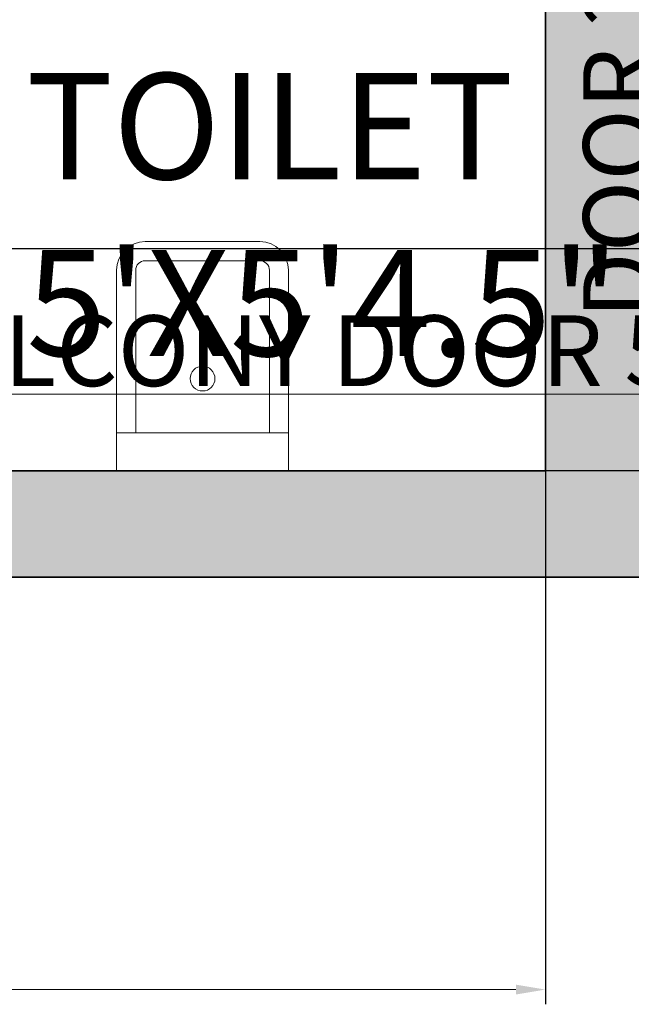
# Model space of a CAD drawing. Units: inches. Extents: x 2696 to 3240, y 1564 to 2310.
# Tile 11 of 76: x 2912 to 2964, y 1569 to 1652. Entities that reach past the tile are written whole.
import ezdxf

# ---------------------------------------------------------------- set-up
doc = ezdxf.new("R2010")
doc.units = ezdxf.units.IN
for name, color, linetype, lineweight in [('A-ANNO-DIMS', 3, 'Continuous', 18), ('A-AREA-IDEN', 7, 'Continuous', 18), ('A-FLOR-FIXT', 8, 'Continuous', 18), ('A-FURN', 251, 'Continuous', 13), ('A-WALL', 7, 'Continuous', 35), ('A-WALL-PATT', 9, 'Continuous', 13)]:
    doc.layers.add(name, color=color, linetype=linetype, lineweight=lineweight)
doc.styles.add('TIMES NEW', font='times.ttf')
doc.styles.add('YQ_DIM', font='SUPEROS.SHX', dxfattribs={"width": 0.8, "bigfont": 'HZDX.SHX'})
doc.dimstyles.new('Siddhuu', dxfattribs={"dimtxt": 6, "dimasz": 2.5, "dimexe": 1.25, "dimexo": 0.625, "dimtad": 1, "dimdec": 1, "dimlunit": 4, "dimtxsty": 'TIMES NEW', "dimcen": 2.5, "dimclrd": 256, "dimclre": 1, "dimclrt": 7, "dimadec": 0, "dimazin": 0, "dimtfac": 1, "dimtdec": 1, "dimtmove": 0, "dimatfit": 3, "dimfxl": 1, "dimtolj": 1, "dimlwd": -1, "dimarcsym": 0})

# ---------------------------------------------------------------- blocks, each defined once
blk = doc.blocks.new('WC')
at = {"layer": 'A-FURN'}
for p, q in [((0, 14.59), (-17.022, 14.59)), ((-3.242, 14.59), (-3.242, 0)), ((-3.242, 12.969), (-17.022, 12.969)), ((-19.454, 2.432), (-19.454, 12.159)), ((-17.833, 2.432), (-17.833, 12.159)), ((-3.242, 1.621), (-17.022, 1.621)), ((0, 0), (-17.022, 0))]:
    blk.add_line(p, q, dxfattribs=at)
blk.add_circle((-7.836, 7.295), 1.051, dxfattribs=at)
for centre, radius, start, end in [((-17.022, 12.159), 2.432, 90, 180), ((-17.022, 12.159), 0.811, 90, 180), ((-17.022, 2.432), 2.432, 180, 270), ((-17.022, 2.432), 0.811, 180, 270)]:
    blk.add_arc(centre, radius, start, end, dxfattribs=at)
blk = doc.blocks.new('*D32')
at = {"layer": 'A-ANNO-DIMS', "color": 1, "lineweight": -2, "transparency": 16777216}
for p, q in [((2962.734, 1723.327), (2967.859, 1723.327)), ((2962.734, 1693.327), (2967.859, 1693.327))]:
    blk.add_line(p, q, dxfattribs=at)
at = {"layer": 'A-ANNO-DIMS', "transparency": 16777216}
for p, q in [((2966.609, 1720.827), (2966.609, 1695.827)), ((2966.609, 1693.327), (2966.609, 1624.849))]:
    blk.add_line(p, q, dxfattribs=at)
for points in [[(2966.192, 1720.827), (2967.025, 1720.827), (2966.609, 1723.327)], [(2966.192, 1695.827), (2967.025, 1695.827), (2966.609, 1693.327)]]:
    blk.add_solid(points, dxfattribs=at)
at = {"layer": 'Defpoints', "color": 0, "transparency": 16777216}
for p in [(2962.109, 1723.327), (2962.109, 1693.327), (2966.609, 1693.327)]:
    blk.add_point(p, dxfattribs=at)
at = {"layer": 'A-ANNO-DIMS', "color": 7, "transparency": 16777216, "insert": (2962.917, 1657.838), "char_height": 6, "attachment_point": 5, "rotation": 90, "style": 'TIMES NEW'}
blk.add_mtext('\\A1;DOOR 2\'-6" TYP.', dxfattribs=at)
blk = doc.blocks.new('*D36')
at = {"layer": 'A-ANNO-DIMS', "color": 1, "lineweight": -2, "transparency": 16777216}
for p, q in [((3008.237, 1629.386), (3008.237, 1619.461)), ((3070.237, 1629.386), (3070.237, 1619.461))]:
    blk.add_line(p, q, dxfattribs=at)
at = {"layer": 'A-ANNO-DIMS', "transparency": 16777216}
for p, q in [((3008.237, 1620.711), (2894.718, 1620.711)), ((3067.737, 1620.711), (3010.737, 1620.711))]:
    blk.add_line(p, q, dxfattribs=at)
for points in [[(3010.737, 1621.128), (3010.737, 1620.294), (3008.237, 1620.711)], [(3067.737, 1621.128), (3067.737, 1620.294), (3070.237, 1620.711)]]:
    blk.add_solid(points, dxfattribs=at)
at = {"layer": 'Defpoints', "color": 0, "transparency": 16777216}
for p in [(3008.237, 1630.011), (3070.237, 1630.011), (3008.237, 1620.711)]:
    blk.add_point(p, dxfattribs=at)
at = {"layer": 'A-ANNO-DIMS', "color": 7, "transparency": 16777216, "insert": (2950.228, 1624.403), "char_height": 6, "attachment_point": 5, "style": 'TIMES NEW'}
blk.add_mtext('\\A1;BALCONY DOOR 5\'-2" TYP.', dxfattribs=at)
blk = doc.blocks.new('*D57')
at = {"layer": 'A-ANNO-DIMS', "color": 1, "lineweight": -2, "transparency": 16777216}
for p, q in [((2754.611, 2018.576), (2754.611, 1568.951)), ((2956.709, 2018.576), (2956.709, 1568.951))]:
    blk.add_line(p, q, dxfattribs=at)
at = {"layer": 'A-ANNO-DIMS', "transparency": 16777216}
blk.add_line((2757.111, 1570.201), (2954.209, 1570.201), dxfattribs=at)
for points in [[(2757.111, 1570.618), (2757.111, 1569.784), (2754.611, 1570.201)], [(2954.209, 1570.618), (2954.209, 1569.784), (2956.709, 1570.201)]]:
    blk.add_solid(points, dxfattribs=at)
at = {"layer": 'Defpoints', "color": 0, "transparency": 16777216}
for p in [(2754.611, 2019.201), (2956.709, 2019.201), (2956.709, 1570.201)]:
    blk.add_point(p, dxfattribs=at)
at = {"layer": 'A-ANNO-DIMS', "color": 7, "transparency": 16777216, "insert": (2855.66, 1573.878), "char_height": 6, "attachment_point": 5, "style": 'TIMES NEW'}
blk.add_mtext('\\A1;16\'-10"', dxfattribs=at)
blk = doc.blocks.new('*D81')
at = {"layer": 'A-ANNO-DIMS', "color": 1, "lineweight": -2, "transparency": 16777216}
for p, q in [((3189.986, 1633.048), (2709.361, 1633.048)), ((3189.986, 1614.201), (2709.361, 1614.201))]:
    blk.add_line(p, q, dxfattribs=at)
at = {"layer": 'A-ANNO-DIMS', "transparency": 16777216}
blk.add_line((2710.611, 1616.701), (2710.611, 1630.548), dxfattribs=at)
for points in [[(2710.195, 1630.548), (2711.028, 1630.548), (2710.611, 1633.048)], [(2710.195, 1616.701), (2711.028, 1616.701), (2710.611, 1614.201)]]:
    blk.add_solid(points, dxfattribs=at)
at = {"layer": 'Defpoints', "color": 0, "transparency": 16777216}
for p in [(2710.611, 1633.048), (3190.611, 1633.048), (3190.611, 1614.201)]:
    blk.add_point(p, dxfattribs=at)
at = {"layer": 'A-ANNO-DIMS', "color": 7, "transparency": 16777216, "insert": (2706.926, 1623.624), "char_height": 6, "attachment_point": 5, "rotation": 90, "style": 'TIMES NEW'}
blk.add_mtext('\\A1;1\'-7"', dxfattribs=at)

msp = doc.modelspace()

# ---------------------------------------------------------------- hatches: boundary and pattern name
at = {"layer": 'A-WALL-PATT', "transparency": 33554556}
h = msp.add_hatch(color=256, dxfattribs=at)
h.dxf.hatch_style = 1
h.paths.add_polyline_path([(2879.111, 2253.201), (2905.91, 2253.201), (2905.91, 2262.201), (2841.889, 2262.201), (2841.889, 2253.201), (2870.111, 2253.201), (2870.111, 2176.601), (2965.709, 2176.601), (2965.709, 2206.701), (2973.583, 2206.701), (2973.583, 2215.701), (2965.709, 2215.701), (2965.709, 2262.201), (2929.91, 2262.201), (2929.91, 2253.201), (2956.709, 2253.201), (2956.709, 2185.601), (2879.111, 2185.601)])
h.paths.add_polyline_path([(2782.834, 2262.201), (2745.611, 2262.201), (2745.611, 2228.729), (2754.611, 2228.729), (2754.611, 2253.201), (2782.834, 2253.201)])
h.paths.add_polyline_path([(2754.611, 2136.201), (2965.709, 2136.201), (2965.709, 2145.201), (2879.111, 2145.201), (2879.111, 2147.074), (2877.34, 2147.074), (2870.111, 2147.074), (2870.111, 2145.201), (2754.611, 2145.201), (2754.611, 2169.674), (2745.611, 2169.674), (2745.611, 2000.201), (2754.611, 2000.201), (2754.611, 2019.201), (2849.083, 2019.201), (2849.083, 2023.701), (2841.209, 2023.701), (2841.209, 2051.827), (2836.709, 2051.827), (2836.709, 2023.701), (2754.611, 2023.701), (2754.611, 2091.201), (2836.709, 2091.201), (2836.709, 2087.827), (2841.209, 2087.827), (2841.209, 2095.701), (2754.611, 2095.701)])
h.paths.add_polyline_path([(2965.709, 2136.201), (2956.709, 2136.201), (2956.709, 2023.701), (2885.083, 2023.701), (2885.083, 2019.201), (2956.709, 2019.201), (2956.709, 1950.575), (2965.709, 1950.575), (2965.709, 1980.201), (2973.583, 1980.201), (2973.583, 1989.201), (2965.709, 1989.201)])
h.paths.add_polyline_path([(2754.611, 1906.701), (2880.209, 1906.701), (2884.709, 1906.701), (2956.709, 1906.701), (2956.709, 1792.701), (2944.709, 1792.701), (2944.709, 1783.701), (2956.709, 1783.701), (2956.709, 1740.201), (2884.709, 1740.201), (2884.709, 1783.701), (2896.709, 1783.701), (2896.709, 1792.701), (2884.709, 1792.701), (2884.709, 1846.701), (2880.209, 1846.701), (2880.209, 1740.201), (2754.611, 1740.201), (2754.611, 1777.201), (2745.611, 1777.201), (2745.611, 1692.701), (2754.611, 1692.701), (2754.611, 1731.201), (2956.709, 1731.201), (2956.709, 1723.327), (2965.709, 1723.327), (2965.709, 1884.201), (2973.583, 1884.201), (2973.583, 1893.201), (2965.709, 1893.201), (2965.709, 1914.575), (2956.709, 1914.575), (2956.709, 1911.201), (2754.611, 1911.201), (2754.611, 1930.201), (2745.611, 1930.201), (2745.611, 1817.201), (2754.611, 1817.201), (2754.611, 1854.201), (2826.611, 1854.201), (2826.611, 1868.827), (2822.111, 1868.827), (2822.111, 1858.701), (2754.611, 1858.701)])
h.paths.add_polyline_path([(2965.709, 1656.201), (3008.237, 1656.201), (3008.237, 1665.201), (2965.709, 1665.201), (2965.709, 1693.327), (2956.709, 1693.327), (2956.709, 1686.201), (2934.583, 1686.201), (2934.583, 1681.701), (2956.709, 1681.701), (2956.709, 1614.201), (2896.709, 1614.201), (2896.709, 1681.701), (2904.583, 1681.701), (2904.583, 1686.201), (2892.209, 1686.201), (2892.209, 1614.201), (2858.41, 1614.201), (2858.41, 1605.201), (2965.709, 1605.201)])
h.paths.add_polyline_path([(2788.41, 1614.201), (2754.611, 1614.201), (2754.611, 1652.701), (2745.611, 1652.701), (2745.611, 1605.201), (2788.41, 1605.201)])
h.paths.add_polyline_path([(3199.611, 1633.048), (3190.611, 1633.048), (3190.611, 1614.201), (3082.611, 1614.201), (3082.611, 1665.201), (3070.237, 1665.201), (3070.237, 1656.201), (3078.111, 1656.201), (3078.111, 1605.201), (3199.611, 1605.201)])
h.paths.add_polyline_path([(3199.611, 1702.048), (3190.611, 1702.048), (3190.611, 1699.701), (3106.611, 1699.701), (3106.611, 1747.701), (3190.611, 1747.701), (3190.611, 1752.201), (3082.611, 1752.201), (3082.611, 1760.075), (3078.111, 1760.075), (3078.111, 1747.701), (3102.111, 1747.701), (3102.111, 1699.701), (3078.111, 1699.701), (3078.111, 1695.201), (3190.611, 1695.201), (3190.611, 1676.355), (3199.611, 1676.355)])
h.paths.add_polyline_path([(3199.611, 1783.201), (3190.611, 1783.201), (3190.611, 1745.355), (3199.611, 1745.355)])
h.paths.add_polyline_path([(3082.611, 1884.201), (3190.611, 1884.201), (3190.611, 1853.201), (3199.611, 1853.201), (3199.611, 1901.701), (3190.611, 1901.701), (3190.611, 1893.201), (3005.583, 1893.201), (3005.583, 1891.281), (3005.583, 1884.201), (3078.111, 1884.201), (3078.111, 1792.075), (3082.611, 1792.075)])
h.paths.add_polyline_path([(3199.611, 1994.701), (3190.611, 1994.701), (3190.611, 1989.201), (3073.709, 1989.201), (3073.709, 2034.201), (3069.209, 2034.201), (3069.209, 1989.201), (3005.583, 1989.201), (3005.583, 1980.201), (3190.611, 1980.201), (3190.611, 1971.701), (3199.611, 1971.701)])
h.paths.add_polyline_path([(3199.611, 2155.201), (3190.611, 2155.201), (3190.611, 2064.701), (3199.611, 2064.701)])
h.paths.add_polyline_path([(3190.611, 2074.701), (3106.611, 2074.701), (3106.611, 2122.701), (3190.611, 2122.701), (3190.611, 2127.201), (3082.709, 2127.201), (3082.709, 2135.075), (3073.709, 2135.075), (3073.709, 2122.701), (3102.111, 2122.701), (3102.111, 2074.701), (3069.209, 2074.701), (3069.209, 2070.201), (3190.611, 2070.201)])
h.paths.add_polyline_path([(3082.709, 2253.201), (3190.611, 2253.201), (3190.611, 2225.201), (3199.611, 2225.201), (3199.611, 2262.201), (3073.709, 2262.201), (3073.709, 2215.701), (3035.583, 2215.701), (3035.583, 2206.701), (3073.709, 2206.701), (3073.709, 2171.075), (3082.709, 2171.075)])

# ---------------------------------------------------------------- linework, layer by layer
at = {"layer": 'A-WALL'}
for p, q in [((2956.709, 1681.701), (2956.709, 1614.201)), ((2896.709, 1614.201), (2956.709, 1614.201)), ((2858.41, 1605.201), (2965.709, 1605.201))]:
    msp.add_line(p, q, dxfattribs=at)

# ---------------------------------------------------------------- block references
at = {"layer": 'A-FLOR-FIXT', "xscale": -1, "rotation": 90}
msp.add_blockref('WC', (2934.922, 1614.201), dxfattribs=at)

# ---------------------------------------------------------------- texts
at = {"layer": 'A-AREA-IDEN', "insert": (2912.674, 1647.951), "char_height": 9, "attachment_point": 1, "style": 'YQ_DIM'}
msp.add_mtext_dynamic_manual_height_columns('TOILET\\P5\'X5\'4.5"', width=48.00324, gutter_width=12.5, heights=[0], dxfattribs=at)

# ---------------------------------------------------------------- dimensions: what is measured, and where the dimension line sits
at = {"layer": 'A-ANNO-DIMS'}
dim = msp.add_linear_dim(base=(2956.709, 1570.201), p1=(2754.611, 2019.201), p2=(2956.709, 2019.201), dimstyle='Siddhuu', override={"dimdec": 1, "dimlfac": 1, "dimrnd": 0, "dimzin": 1, "dimdsep": 46, "dimlunit": 4, "dimfrac": 2}, dxfattribs=at)
dim.commit()
dim.dimension.update_dxf_attribs({"geometry": '*D57', "text_midpoint": (2855.66, 1573.878)})
for base, p1, p2, angle, text, picture, middle in [((2966.609, 1693.327), (2962.109, 1723.327), (2962.109, 1693.327), 270, 'DOOR <> TYP.', '*D32', (2962.917, 1657.838)), ((3008.237, 1620.711), (3070.237, 1630.011), (3008.237, 1630.011), 180, 'BALCONY DOOR <> TYP.', '*D36', (2950.228, 1624.403))]:
    dim = msp.add_linear_dim(base=base, p1=p1, p2=p2, angle=angle, text=text, dimstyle='Siddhuu', override={"dimdec": 1, "dimlfac": 1, "dimrnd": 0, "dimzin": 1, "dimdsep": 46, "dimlunit": 4, "dimfrac": 2}, dxfattribs=at)
    dim.commit()
    dim.dimension.update_dxf_attribs({"geometry": picture, "text_midpoint": middle})
dim = msp.add_linear_dim(base=(2710.611, 1633.048), p1=(3190.611, 1614.201), p2=(3190.611, 1633.048), angle=90, dimstyle='Siddhuu', override={"dimdec": 1, "dimlfac": 1, "dimrnd": 0, "dimzin": 1, "dimdsep": 46, "dimlunit": 4, "dimfrac": 2}, dxfattribs=at)
dim.commit()
dim.dimension.update_dxf_attribs({"geometry": '*D81', "text_midpoint": (2706.926, 1623.624)})

doc.saveas('drawing.dxf')
